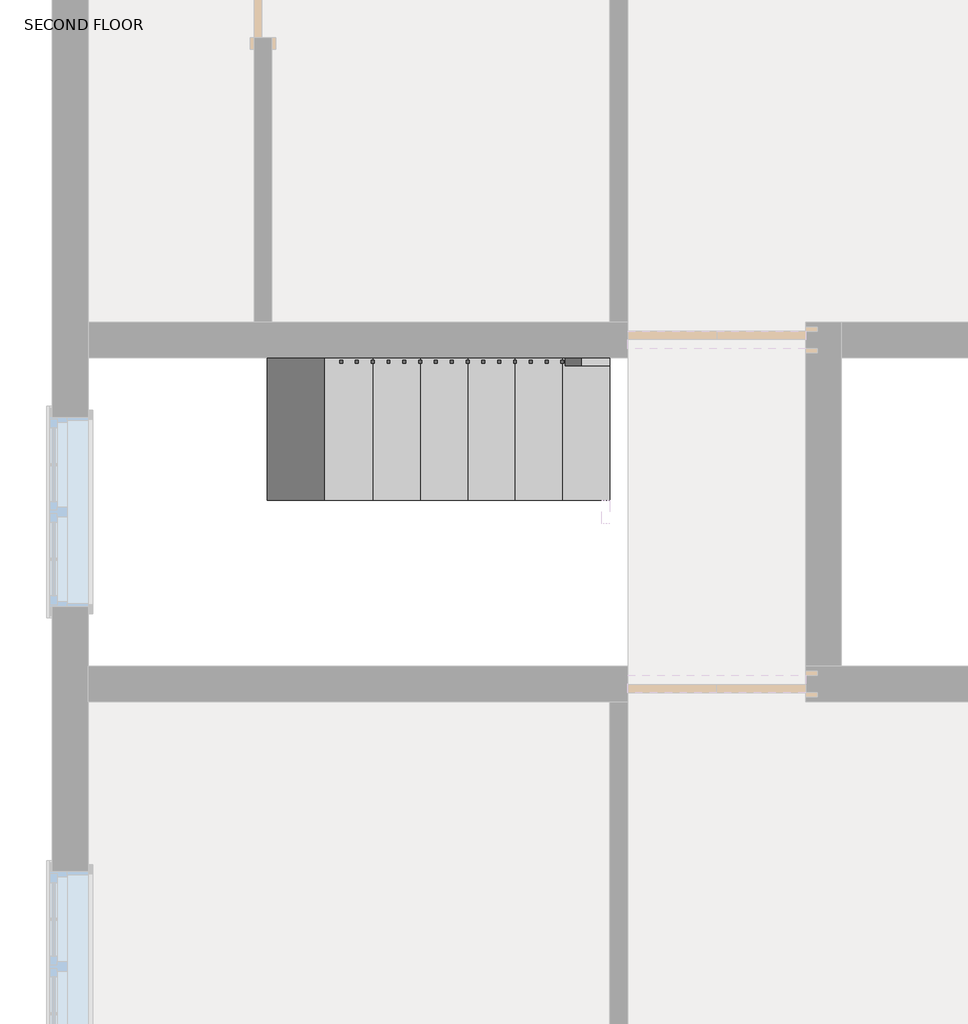
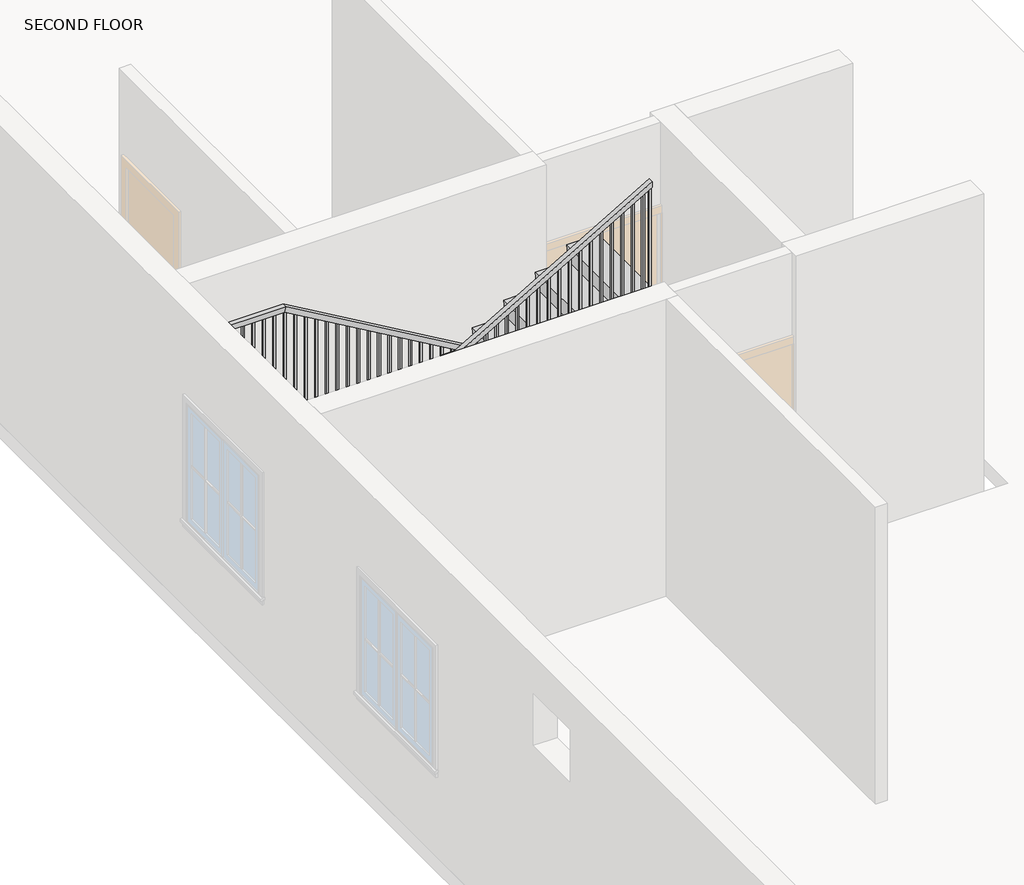
# One storey, part 3 of 4: 1 railing, 1 stair flight.
"""IFC4 building model written with IfcOpenShell, lengths in millimetres."""

from ifc_helpers import new_model, si_unit, frame, origin, place, context, project, spatial, polyline, outline, extrude, faceted_brep, element, save

model = new_model("IFC4")

# Units and contexts
model_context = context("Model", 3, world=origin())
ifc_project = project(units=[si_unit("LENGTHUNIT", "METRE", prefix="MILLI")], contexts=[model_context])

# Site, building, storey
site = spatial("IfcSite", under=ifc_project)
building = spatial("IfcBuilding", under=site)
storey = spatial("IfcBuildingStorey", under=building, Name="SECOND FLOOR", Elevation=6400.8)

# Railing
placement = place(None, origin())
element("IfcRailing", 1, ObjectType="Handrail - Rectangular", at=placement, inside=storey, context=model_context, shape_type="SolidModel", body=[
    faceted_brep([(-2776.8289041, 1499.0153263, 7493.0), (-2776.8289041, 1499.0153263, 7434.1886538), (-2776.8289041, 1549.8153263, 7434.1886538), (-2776.8289041, 1549.8153263, 7493.0), (-5215.2289041, 1499.0153263, 8915.4), (-5228.9626405, 1499.0153263, 8864.6), (-5228.9626405, 1549.8153263, 8864.6), (-5215.2289041, 1549.8153263, 8915.4), (-6078.8289041, 1499.0153263, 8915.4), (-6078.8289041, 1499.0153263, 8864.6), (-6129.6289041, 1549.8153263, 8864.6), (-6129.6289041, 1549.8153263, 8915.4), (-6078.8289041, -380.5846737, 8915.4), (-6078.8289041, -380.5846737, 8864.6), (-6129.6289041, -431.3846737, 8864.6), (-6129.6289041, -431.3846737, 8915.4), (-5520.0289041, -380.5846737, 8915.4), (-5506.2951677, -380.5846737, 8864.6), (-5506.2951677, -431.3846737, 8864.6), (-5520.0289041, -431.3846737, 8915.4), (-2776.8289041, -380.5846737, 10515.6), (-2776.8289041, -431.3846737, 10515.6), (-2776.8289041, -431.3846737, 10456.7886538), (-2776.8289041, -380.5846737, 10456.7886538)], [[[0, 1, 2, 3]], [[1, 0, 4, 5]], [[2, 1, 5, 6]], [[3, 2, 6, 7]], [[0, 3, 7, 4]], [[5, 4, 8, 9]], [[6, 5, 9, 10]], [[7, 6, 10, 11]], [[4, 7, 11, 8]], [[9, 8, 12, 13]], [[10, 9, 13, 14]], [[11, 10, 14, 15]], [[8, 11, 15, 12]], [[13, 12, 16, 17]], [[14, 13, 17, 18]], [[15, 14, 18, 19]], [[12, 15, 19, 16]], [[20, 21, 22, 23]], [[17, 16, 20, 23]], [[18, 17, 23, 22]], [[19, 18, 22, 21]], [[16, 19, 21, 20]]]),
    extrude(outline(polyline([(10417.8949038, -2843.5039041), (10406.7824038, -2862.5539041), (9423.4, -2862.5539041), (9423.4, -2843.5039041), (10417.8949038, -2843.5039041)])), frame((0.0, -415.5096737, 0.0), z_axis=(0.0, 1.0, 0.0), x_axis=(0.0, 0.0, 1.0)), (0.0, 0.0, 1.0), 19.05),
    extrude(outline(polyline([(10358.6282371, -2945.1039041), (10347.5157371, -2964.1539041), (9423.4, -2964.1539041), (9423.4, -2945.1039041), (10358.6282371, -2945.1039041)])), frame((0.0, -415.5096737, 0.0), z_axis=(0.0, 1.0, 0.0), x_axis=(0.0, 0.0, 1.0)), (0.0, 0.0, 1.0), 19.05),
    extrude(outline(polyline([(10299.3615704, -3046.7039041), (10288.2490704, -3065.7539041), (9423.4, -3065.7539041), (9423.4, -3046.7039041), (10299.3615704, -3046.7039041)])), frame((0.0, -415.5096737, 0.0), z_axis=(0.0, 1.0, 0.0), x_axis=(0.0, 0.0, 1.0)), (0.0, 0.0, 1.0), 19.05),
    extrude(outline(polyline([(10240.0949038, -3148.3039041), (10228.9824038, -3167.3539041), (9245.6, -3167.3539041), (9245.6, -3148.3039041), (10240.0949038, -3148.3039041)])), frame((0.0, -415.5096737, 0.0), z_axis=(0.0, 1.0, 0.0), x_axis=(0.0, 0.0, 1.0)), (0.0, 0.0, 1.0), 19.05),
    extrude(outline(polyline([(10180.8282371, -3249.9039041), (10169.7157371, -3268.9539041), (9245.6, -3268.9539041), (9245.6, -3249.9039041), (10180.8282371, -3249.9039041)])), frame((0.0, -415.5096737, 0.0), z_axis=(0.0, 1.0, 0.0), x_axis=(0.0, 0.0, 1.0)), (0.0, 0.0, 1.0), 19.05),
    extrude(outline(polyline([(10121.5615704, -3351.5039041), (10110.4490704, -3370.5539041), (9245.6, -3370.5539041), (9245.6, -3351.5039041), (10121.5615704, -3351.5039041)])), frame((0.0, -415.5096737, 0.0), z_axis=(0.0, 1.0, 0.0), x_axis=(0.0, 0.0, 1.0)), (0.0, 0.0, 1.0), 19.05),
    extrude(outline(polyline([(10062.2949038, -3453.1039041), (10051.1824038, -3472.1539041), (9067.8, -3472.1539041), (9067.8, -3453.1039041), (10062.2949038, -3453.1039041)])), frame((0.0, -415.5096737, 0.0), z_axis=(0.0, 1.0, 0.0), x_axis=(0.0, 0.0, 1.0)), (0.0, 0.0, 1.0), 19.05),
    extrude(outline(polyline([(10003.0282371, -3554.7039041), (9991.9157371, -3573.7539041), (9067.8, -3573.7539041), (9067.8, -3554.7039041), (10003.0282371, -3554.7039041)])), frame((0.0, -415.5096737, 0.0), z_axis=(0.0, 1.0, 0.0), x_axis=(0.0, 0.0, 1.0)), (0.0, 0.0, 1.0), 19.05),
    extrude(outline(polyline([(9943.7615704, -3656.3039041), (9932.6490704, -3675.3539041), (9067.8, -3675.3539041), (9067.8, -3656.3039041), (9943.7615704, -3656.3039041)])), frame((0.0, -415.5096737, 0.0), z_axis=(0.0, 1.0, 0.0), x_axis=(0.0, 0.0, 1.0)), (0.0, 0.0, 1.0), 19.05),
    extrude(outline(polyline([(9884.4949038, -3757.9039041), (9873.3824038, -3776.9539041), (8890.0, -3776.9539041), (8890.0, -3757.9039041), (9884.4949038, -3757.9039041)])), frame((0.0, -415.5096737, 0.0), z_axis=(0.0, 1.0, 0.0), x_axis=(0.0, 0.0, 1.0)), (0.0, 0.0, 1.0), 19.05),
    extrude(outline(polyline([(9825.2282371, -3859.5039041), (9814.1157371, -3878.5539041), (8890.0, -3878.5539041), (8890.0, -3859.5039041), (9825.2282371, -3859.5039041)])), frame((0.0, -415.5096737, 0.0), z_axis=(0.0, 1.0, 0.0), x_axis=(0.0, 0.0, 1.0)), (0.0, 0.0, 1.0), 19.05),
    extrude(outline(polyline([(9765.9615704, -3961.1039041), (9754.8490704, -3980.1539041), (8890.0, -3980.1539041), (8890.0, -3961.1039041), (9765.9615704, -3961.1039041)])), frame((0.0, -415.5096737, 0.0), z_axis=(0.0, 1.0, 0.0), x_axis=(0.0, 0.0, 1.0)), (0.0, 0.0, 1.0), 19.05),
    extrude(outline(polyline([(9706.6949038, -4062.7039041), (9695.5824038, -4081.7539041), (8712.2, -4081.7539041), (8712.2, -4062.7039041), (9706.6949038, -4062.7039041)])), frame((0.0, -415.5096737, 0.0), z_axis=(0.0, 1.0, 0.0), x_axis=(0.0, 0.0, 1.0)), (0.0, 0.0, 1.0), 19.05),
    extrude(outline(polyline([(9647.4282371, -4164.3039041), (9636.3157371, -4183.3539041), (8712.2, -4183.3539041), (8712.2, -4164.3039041), (9647.4282371, -4164.3039041)])), frame((0.0, -415.5096737, 0.0), z_axis=(0.0, 1.0, 0.0), x_axis=(0.0, 0.0, 1.0)), (0.0, 0.0, 1.0), 19.05),
    extrude(outline(polyline([(9588.1615704, -4265.9039041), (9577.0490704, -4284.9539041), (8712.2, -4284.9539041), (8712.2, -4265.9039041), (9588.1615704, -4265.9039041)])), frame((0.0, -415.5096737, 0.0), z_axis=(0.0, 1.0, 0.0), x_axis=(0.0, 0.0, 1.0)), (0.0, 0.0, 1.0), 19.05),
    extrude(outline(polyline([(9528.8949038, -4367.5039041), (9517.7824038, -4386.5539041), (8534.4, -4386.5539041), (8534.4, -4367.5039041), (9528.8949038, -4367.5039041)])), frame((0.0, -415.5096737, 0.0), z_axis=(0.0, 1.0, 0.0), x_axis=(0.0, 0.0, 1.0)), (0.0, 0.0, 1.0), 19.05),
    extrude(outline(polyline([(9469.6282371, -4469.1039041), (9458.5157371, -4488.1539041), (8534.4, -4488.1539041), (8534.4, -4469.1039041), (9469.6282371, -4469.1039041)])), frame((0.0, -415.5096737, 0.0), z_axis=(0.0, 1.0, 0.0), x_axis=(0.0, 0.0, 1.0)), (0.0, 0.0, 1.0), 19.05),
    extrude(outline(polyline([(9410.3615704, -4570.7039041), (9399.2490704, -4589.7539041), (8534.4, -4589.7539041), (8534.4, -4570.7039041), (9410.3615704, -4570.7039041)])), frame((0.0, -415.5096737, 0.0), z_axis=(0.0, 1.0, 0.0), x_axis=(0.0, 0.0, 1.0)), (0.0, 0.0, 1.0), 19.05),
    extrude(outline(polyline([(9351.0949038, -4672.3039041), (9339.9824038, -4691.3539041), (8356.6, -4691.3539041), (8356.6, -4672.3039041), (9351.0949038, -4672.3039041)])), frame((0.0, -415.5096737, 0.0), z_axis=(0.0, 1.0, 0.0), x_axis=(0.0, 0.0, 1.0)), (0.0, 0.0, 1.0), 19.05),
    extrude(outline(polyline([(9291.8282371, -4773.9039041), (9280.7157371, -4792.9539041), (8356.6, -4792.9539041), (8356.6, -4773.9039041), (9291.8282371, -4773.9039041)])), frame((0.0, -415.5096737, 0.0), z_axis=(0.0, 1.0, 0.0), x_axis=(0.0, 0.0, 1.0)), (0.0, 0.0, 1.0), 19.05),
    extrude(outline(polyline([(9232.5615704, -4875.5039041), (9221.4490704, -4894.5539041), (8356.6, -4894.5539041), (8356.6, -4875.5039041), (9232.5615704, -4875.5039041)])), frame((0.0, -415.5096737, 0.0), z_axis=(0.0, 1.0, 0.0), x_axis=(0.0, 0.0, 1.0)), (0.0, 0.0, 1.0), 19.05),
    extrude(outline(polyline([(9173.2949038, -4977.1039041), (9162.1824038, -4996.1539041), (8178.8, -4996.1539041), (8178.8, -4977.1039041), (9173.2949038, -4977.1039041)])), frame((0.0, -415.5096737, 0.0), z_axis=(0.0, 1.0, 0.0), x_axis=(0.0, 0.0, 1.0)), (0.0, 0.0, 1.0), 19.05),
    extrude(outline(polyline([(9114.0282371, -5078.7039041), (9102.9157371, -5097.7539041), (8178.8, -5097.7539041), (8178.8, -5078.7039041), (9114.0282371, -5078.7039041)])), frame((0.0, -415.5096737, 0.0), z_axis=(0.0, 1.0, 0.0), x_axis=(0.0, 0.0, 1.0)), (0.0, 0.0, 1.0), 19.05),
    extrude(outline(polyline([(9054.7615704, -5180.3039041), (9043.6490704, -5199.3539041), (8178.8, -5199.3539041), (8178.8, -5180.3039041), (9054.7615704, -5180.3039041)])), frame((0.0, -415.5096737, 0.0), z_axis=(0.0, 1.0, 0.0), x_axis=(0.0, 0.0, 1.0)), (0.0, 0.0, 1.0), 19.05),
    extrude(outline(polyline([(8995.4949038, -5281.9039041), (8984.3824038, -5300.9539041), (8001.0, -5300.9539041), (8001.0, -5281.9039041), (8995.4949038, -5281.9039041)])), frame((0.0, -415.5096737, 0.0), z_axis=(0.0, 1.0, 0.0), x_axis=(0.0, 0.0, 1.0)), (0.0, 0.0, 1.0), 19.05),
    extrude(outline(polyline([(8936.2282371, -5383.5039041), (8925.1157371, -5402.5539041), (8001.0, -5402.5539041), (8001.0, -5383.5039041), (8936.2282371, -5383.5039041)])), frame((0.0, -415.5096737, 0.0), z_axis=(0.0, 1.0, 0.0), x_axis=(0.0, 0.0, 1.0)), (0.0, 0.0, 1.0), 19.05),
    extrude(outline(polyline([(8876.9615704, -5485.1039041), (8865.8490704, -5504.1539041), (8001.0, -5504.1539041), (8001.0, -5485.1039041), (8876.9615704, -5485.1039041)])), frame((0.0, -415.5096737, 0.0), z_axis=(0.0, 1.0, 0.0), x_axis=(0.0, 0.0, 1.0)), (0.0, 0.0, 1.0), 19.05),
    extrude(outline(polyline([(-5605.7539041, -415.5096737), (-5605.7539041, -396.4596737), (-5586.7039041, -396.4596737), (-5586.7039041, -415.5096737), (-5605.7539041, -415.5096737)])), frame((0.0, 0.0, 8001.0), z_axis=(0.0, 0.0, 1.0), x_axis=(1.0, 0.0, 0.0)), (0.0, 0.0, 1.0), 863.6),
    extrude(outline(polyline([(-5707.3539041, -415.5096737), (-5707.3539041, -396.4596737), (-5688.3039041, -396.4596737), (-5688.3039041, -415.5096737), (-5707.3539041, -415.5096737)])), frame((0.0, 0.0, 8001.0), z_axis=(0.0, 0.0, 1.0), x_axis=(1.0, 0.0, 0.0)), (0.0, 0.0, 1.0), 863.6),
    extrude(outline(polyline([(-5808.9539041, -415.5096737), (-5808.9539041, -396.4596737), (-5789.9039041, -396.4596737), (-5789.9039041, -415.5096737), (-5808.9539041, -415.5096737)])), frame((0.0, 0.0, 8001.0), z_axis=(0.0, 0.0, 1.0), x_axis=(1.0, 0.0, 0.0)), (0.0, 0.0, 1.0), 863.6),
    extrude(outline(polyline([(-5910.5539041, -415.5096737), (-5910.5539041, -396.4596737), (-5891.5039041, -396.4596737), (-5891.5039041, -415.5096737), (-5910.5539041, -415.5096737)])), frame((0.0, 0.0, 8001.0), z_axis=(0.0, 0.0, 1.0), x_axis=(1.0, 0.0, 0.0)), (0.0, 0.0, 1.0), 863.6),
    extrude(outline(polyline([(-6012.1539041, -415.5096737), (-6012.1539041, -396.4596737), (-5993.1039041, -396.4596737), (-5993.1039041, -415.5096737), (-6012.1539041, -415.5096737)])), frame((0.0, 0.0, 8001.0), z_axis=(0.0, 0.0, 1.0), x_axis=(1.0, 0.0, 0.0)), (0.0, 0.0, 1.0), 863.6),
    extrude(outline(polyline([(-6113.7539041, -294.8596737), (-6094.7039041, -294.8596737), (-6094.7039041, -313.9096737), (-6113.7539041, -313.9096737), (-6113.7539041, -294.8596737)])), frame((0.0, 0.0, 8001.0), z_axis=(0.0, 0.0, 1.0), x_axis=(1.0, 0.0, 0.0)), (0.0, 0.0, 1.0), 863.6),
    extrude(outline(polyline([(-6113.7539041, -193.2596737), (-6094.7039041, -193.2596737), (-6094.7039041, -212.3096737), (-6113.7539041, -212.3096737), (-6113.7539041, -193.2596737)])), frame((0.0, 0.0, 8001.0), z_axis=(0.0, 0.0, 1.0), x_axis=(1.0, 0.0, 0.0)), (0.0, 0.0, 1.0), 863.6),
    extrude(outline(polyline([(-6113.7539041, -91.6596737), (-6094.7039041, -91.6596737), (-6094.7039041, -110.7096737), (-6113.7539041, -110.7096737), (-6113.7539041, -91.6596737)])), frame((0.0, 0.0, 8001.0), z_axis=(0.0, 0.0, 1.0), x_axis=(1.0, 0.0, 0.0)), (0.0, 0.0, 1.0), 863.6),
    extrude(outline(polyline([(-6113.7539041, 9.9403263), (-6094.7039041, 9.9403263), (-6094.7039041, -9.1096737), (-6113.7539041, -9.1096737), (-6113.7539041, 9.9403263)])), frame((0.0, 0.0, 8001.0), z_axis=(0.0, 0.0, 1.0), x_axis=(1.0, 0.0, 0.0)), (0.0, 0.0, 1.0), 863.6),
    extrude(outline(polyline([(-6113.7539041, 111.5403263), (-6094.7039041, 111.5403263), (-6094.7039041, 92.4903263), (-6113.7539041, 92.4903263), (-6113.7539041, 111.5403263)])), frame((0.0, 0.0, 8001.0), z_axis=(0.0, 0.0, 1.0), x_axis=(1.0, 0.0, 0.0)), (0.0, 0.0, 1.0), 863.6),
    extrude(outline(polyline([(-6113.7539041, 213.1403263), (-6094.7039041, 213.1403263), (-6094.7039041, 194.0903263), (-6113.7539041, 194.0903263), (-6113.7539041, 213.1403263)])), frame((0.0, 0.0, 8001.0), z_axis=(0.0, 0.0, 1.0), x_axis=(1.0, 0.0, 0.0)), (0.0, 0.0, 1.0), 863.6),
    extrude(outline(polyline([(-6113.7539041, 314.7403263), (-6094.7039041, 314.7403263), (-6094.7039041, 295.6903263), (-6113.7539041, 295.6903263), (-6113.7539041, 314.7403263)])), frame((0.0, 0.0, 8001.0), z_axis=(0.0, 0.0, 1.0), x_axis=(1.0, 0.0, 0.0)), (0.0, 0.0, 1.0), 863.6),
    extrude(outline(polyline([(-6113.7539041, 416.3403263), (-6094.7039041, 416.3403263), (-6094.7039041, 397.2903263), (-6113.7539041, 397.2903263), (-6113.7539041, 416.3403263)])), frame((0.0, 0.0, 8001.0), z_axis=(0.0, 0.0, 1.0), x_axis=(1.0, 0.0, 0.0)), (0.0, 0.0, 1.0), 863.6),
    extrude(outline(polyline([(-6113.7539041, 517.9403263), (-6094.7039041, 517.9403263), (-6094.7039041, 498.8903263), (-6113.7539041, 498.8903263), (-6113.7539041, 517.9403263)])), frame((0.0, 0.0, 8001.0), z_axis=(0.0, 0.0, 1.0), x_axis=(1.0, 0.0, 0.0)), (0.0, 0.0, 1.0), 863.6),
    extrude(outline(polyline([(-6113.7539041, 619.5403263), (-6094.7039041, 619.5403263), (-6094.7039041, 600.4903263), (-6113.7539041, 600.4903263), (-6113.7539041, 619.5403263)])), frame((0.0, 0.0, 8001.0), z_axis=(0.0, 0.0, 1.0), x_axis=(1.0, 0.0, 0.0)), (0.0, 0.0, 1.0), 863.6),
    extrude(outline(polyline([(-6113.7539041, 721.1403263), (-6094.7039041, 721.1403263), (-6094.7039041, 702.0903263), (-6113.7539041, 702.0903263), (-6113.7539041, 721.1403263)])), frame((0.0, 0.0, 8001.0), z_axis=(0.0, 0.0, 1.0), x_axis=(1.0, 0.0, 0.0)), (0.0, 0.0, 1.0), 863.6),
    extrude(outline(polyline([(-6113.7539041, 822.7403263), (-6094.7039041, 822.7403263), (-6094.7039041, 803.6903263), (-6113.7539041, 803.6903263), (-6113.7539041, 822.7403263)])), frame((0.0, 0.0, 8001.0), z_axis=(0.0, 0.0, 1.0), x_axis=(1.0, 0.0, 0.0)), (0.0, 0.0, 1.0), 863.6),
    extrude(outline(polyline([(-6113.7539041, 924.3403263), (-6094.7039041, 924.3403263), (-6094.7039041, 905.2903263), (-6113.7539041, 905.2903263), (-6113.7539041, 924.3403263)])), frame((0.0, 0.0, 8001.0), z_axis=(0.0, 0.0, 1.0), x_axis=(1.0, 0.0, 0.0)), (0.0, 0.0, 1.0), 863.6),
    extrude(outline(polyline([(-6113.7539041, 1025.9403263), (-6094.7039041, 1025.9403263), (-6094.7039041, 1006.8903263), (-6113.7539041, 1006.8903263), (-6113.7539041, 1025.9403263)])), frame((0.0, 0.0, 8001.0), z_axis=(0.0, 0.0, 1.0), x_axis=(1.0, 0.0, 0.0)), (0.0, 0.0, 1.0), 863.6),
    extrude(outline(polyline([(-6113.7539041, 1127.5403263), (-6094.7039041, 1127.5403263), (-6094.7039041, 1108.4903263), (-6113.7539041, 1108.4903263), (-6113.7539041, 1127.5403263)])), frame((0.0, 0.0, 8001.0), z_axis=(0.0, 0.0, 1.0), x_axis=(1.0, 0.0, 0.0)), (0.0, 0.0, 1.0), 863.6),
    extrude(outline(polyline([(-6113.7539041, 1229.1403263), (-6094.7039041, 1229.1403263), (-6094.7039041, 1210.0903263), (-6113.7539041, 1210.0903263), (-6113.7539041, 1229.1403263)])), frame((0.0, 0.0, 8001.0), z_axis=(0.0, 0.0, 1.0), x_axis=(1.0, 0.0, 0.0)), (0.0, 0.0, 1.0), 863.6),
    extrude(outline(polyline([(-6113.7539041, 1330.7403263), (-6094.7039041, 1330.7403263), (-6094.7039041, 1311.6903263), (-6113.7539041, 1311.6903263), (-6113.7539041, 1330.7403263)])), frame((0.0, 0.0, 8001.0), z_axis=(0.0, 0.0, 1.0), x_axis=(1.0, 0.0, 0.0)), (0.0, 0.0, 1.0), 863.6),
    extrude(outline(polyline([(-6113.7539041, 1432.3403263), (-6094.7039041, 1432.3403263), (-6094.7039041, 1413.2903263), (-6113.7539041, 1413.2903263), (-6113.7539041, 1432.3403263)])), frame((0.0, 0.0, 8001.0), z_axis=(0.0, 0.0, 1.0), x_axis=(1.0, 0.0, 0.0)), (0.0, 0.0, 1.0), 863.6),
    extrude(outline(polyline([(-6018.5039041, 1533.9403263), (-6018.5039041, 1514.8903263), (-6037.5539041, 1514.8903263), (-6037.5539041, 1533.9403263), (-6018.5039041, 1533.9403263)])), frame((0.0, 0.0, 8001.0), z_axis=(0.0, 0.0, 1.0), x_axis=(1.0, 0.0, 0.0)), (0.0, 0.0, 1.0), 863.6),
    extrude(outline(polyline([(-5916.9039041, 1533.9403263), (-5916.9039041, 1514.8903263), (-5935.9539041, 1514.8903263), (-5935.9539041, 1533.9403263), (-5916.9039041, 1533.9403263)])), frame((0.0, 0.0, 8001.0), z_axis=(0.0, 0.0, 1.0), x_axis=(1.0, 0.0, 0.0)), (0.0, 0.0, 1.0), 863.6),
    extrude(outline(polyline([(-5815.3039041, 1533.9403263), (-5815.3039041, 1514.8903263), (-5834.3539041, 1514.8903263), (-5834.3539041, 1533.9403263), (-5815.3039041, 1533.9403263)])), frame((0.0, 0.0, 8001.0), z_axis=(0.0, 0.0, 1.0), x_axis=(1.0, 0.0, 0.0)), (0.0, 0.0, 1.0), 863.6),
    extrude(outline(polyline([(-5713.7039041, 1533.9403263), (-5713.7039041, 1514.8903263), (-5732.7539041, 1514.8903263), (-5732.7539041, 1533.9403263), (-5713.7039041, 1533.9403263)])), frame((0.0, 0.0, 8001.0), z_axis=(0.0, 0.0, 1.0), x_axis=(1.0, 0.0, 0.0)), (0.0, 0.0, 1.0), 863.6),
    extrude(outline(polyline([(-5612.1039041, 1533.9403263), (-5612.1039041, 1514.8903263), (-5631.1539041, 1514.8903263), (-5631.1539041, 1533.9403263), (-5612.1039041, 1533.9403263)])), frame((0.0, 0.0, 8001.0), z_axis=(0.0, 0.0, 1.0), x_axis=(1.0, 0.0, 0.0)), (0.0, 0.0, 1.0), 863.6),
    extrude(outline(polyline([(-5510.5039041, 1533.9403263), (-5510.5039041, 1514.8903263), (-5529.5539041, 1514.8903263), (-5529.5539041, 1533.9403263), (-5510.5039041, 1533.9403263)])), frame((0.0, 0.0, 8001.0), z_axis=(0.0, 0.0, 1.0), x_axis=(1.0, 0.0, 0.0)), (0.0, 0.0, 1.0), 863.6),
    extrude(outline(polyline([(-5408.9039041, 1533.9403263), (-5408.9039041, 1514.8903263), (-5427.9539041, 1514.8903263), (-5427.9539041, 1533.9403263), (-5408.9039041, 1533.9403263)])), frame((0.0, 0.0, 8001.0), z_axis=(0.0, 0.0, 1.0), x_axis=(1.0, 0.0, 0.0)), (0.0, 0.0, 1.0), 863.6),
    extrude(outline(polyline([(-5307.3039041, 1533.9403263), (-5307.3039041, 1514.8903263), (-5326.3539041, 1514.8903263), (-5326.3539041, 1533.9403263), (-5307.3039041, 1533.9403263)])), frame((0.0, 0.0, 8001.0), z_axis=(0.0, 0.0, 1.0), x_axis=(1.0, 0.0, 0.0)), (0.0, 0.0, 1.0), 863.6),
    extrude(outline(polyline([(8851.0324038, -5205.7039041), (8862.1449038, -5224.7539041), (8001.0, -5224.7539041), (8001.0, -5205.7039041), (8851.0324038, -5205.7039041)])), frame((0.0, 1514.8903263, 0.0), z_axis=(0.0, 1.0, 0.0), x_axis=(0.0, 0.0, 1.0)), (0.0, 0.0, 1.0), 19.05),
    extrude(outline(polyline([(8791.7657371, -5104.1039041), (8802.8782371, -5123.1539041), (7823.2, -5123.1539041), (7823.2, -5104.1039041), (8791.7657371, -5104.1039041)])), frame((0.0, 1514.8903263, 0.0), z_axis=(0.0, 1.0, 0.0), x_axis=(0.0, 0.0, 1.0)), (0.0, 0.0, 1.0), 19.05),
    extrude(outline(polyline([(8732.4990704, -5002.5039041), (8743.6115704, -5021.5539041), (7823.2, -5021.5539041), (7823.2, -5002.5039041), (8732.4990704, -5002.5039041)])), frame((0.0, 1514.8903263, 0.0), z_axis=(0.0, 1.0, 0.0), x_axis=(0.0, 0.0, 1.0)), (0.0, 0.0, 1.0), 19.05),
    extrude(outline(polyline([(8673.2324038, -4900.9039041), (8684.3449038, -4919.9539041), (7823.2, -4919.9539041), (7823.2, -4900.9039041), (8673.2324038, -4900.9039041)])), frame((0.0, 1514.8903263, 0.0), z_axis=(0.0, 1.0, 0.0), x_axis=(0.0, 0.0, 1.0)), (0.0, 0.0, 1.0), 19.05),
    extrude(outline(polyline([(8613.9657371, -4799.3039041), (8625.0782371, -4818.3539041), (7645.4, -4818.3539041), (7645.4, -4799.3039041), (8613.9657371, -4799.3039041)])), frame((0.0, 1514.8903263, 0.0), z_axis=(0.0, 1.0, 0.0), x_axis=(0.0, 0.0, 1.0)), (0.0, 0.0, 1.0), 19.05),
    extrude(outline(polyline([(8554.6990704, -4697.7039041), (8565.8115704, -4716.7539041), (7645.4, -4716.7539041), (7645.4, -4697.7039041), (8554.6990704, -4697.7039041)])), frame((0.0, 1514.8903263, 0.0), z_axis=(0.0, 1.0, 0.0), x_axis=(0.0, 0.0, 1.0)), (0.0, 0.0, 1.0), 19.05),
    extrude(outline(polyline([(8495.4324038, -4596.1039041), (8506.5449038, -4615.1539041), (7645.4, -4615.1539041), (7645.4, -4596.1039041), (8495.4324038, -4596.1039041)])), frame((0.0, 1514.8903263, 0.0), z_axis=(0.0, 1.0, 0.0), x_axis=(0.0, 0.0, 1.0)), (0.0, 0.0, 1.0), 19.05),
    extrude(outline(polyline([(8436.1657371, -4494.5039041), (8447.2782371, -4513.5539041), (7467.6, -4513.5539041), (7467.6, -4494.5039041), (8436.1657371, -4494.5039041)])), frame((0.0, 1514.8903263, 0.0), z_axis=(0.0, 1.0, 0.0), x_axis=(0.0, 0.0, 1.0)), (0.0, 0.0, 1.0), 19.05),
    extrude(outline(polyline([(8376.8990704, -4392.9039041), (8388.0115704, -4411.9539041), (7467.6, -4411.9539041), (7467.6, -4392.9039041), (8376.8990704, -4392.9039041)])), frame((0.0, 1514.8903263, 0.0), z_axis=(0.0, 1.0, 0.0), x_axis=(0.0, 0.0, 1.0)), (0.0, 0.0, 1.0), 19.05),
    extrude(outline(polyline([(8317.6324038, -4291.3039041), (8328.7449038, -4310.3539041), (7467.6, -4310.3539041), (7467.6, -4291.3039041), (8317.6324038, -4291.3039041)])), frame((0.0, 1514.8903263, 0.0), z_axis=(0.0, 1.0, 0.0), x_axis=(0.0, 0.0, 1.0)), (0.0, 0.0, 1.0), 19.05),
    extrude(outline(polyline([(8258.3657371, -4189.7039041), (8269.4782371, -4208.7539041), (7289.8, -4208.7539041), (7289.8, -4189.7039041), (8258.3657371, -4189.7039041)])), frame((0.0, 1514.8903263, 0.0), z_axis=(0.0, 1.0, 0.0), x_axis=(0.0, 0.0, 1.0)), (0.0, 0.0, 1.0), 19.05),
    extrude(outline(polyline([(8199.0990704, -4088.1039041), (8210.2115704, -4107.1539041), (7289.8, -4107.1539041), (7289.8, -4088.1039041), (8199.0990704, -4088.1039041)])), frame((0.0, 1514.8903263, 0.0), z_axis=(0.0, 1.0, 0.0), x_axis=(0.0, 0.0, 1.0)), (0.0, 0.0, 1.0), 19.05),
    extrude(outline(polyline([(8139.8324038, -3986.5039041), (8150.9449038, -4005.5539041), (7289.8, -4005.5539041), (7289.8, -3986.5039041), (8139.8324038, -3986.5039041)])), frame((0.0, 1514.8903263, 0.0), z_axis=(0.0, 1.0, 0.0), x_axis=(0.0, 0.0, 1.0)), (0.0, 0.0, 1.0), 19.05),
    extrude(outline(polyline([(8080.5657371, -3884.9039041), (8091.6782371, -3903.9539041), (7112.0, -3903.9539041), (7112.0, -3884.9039041), (8080.5657371, -3884.9039041)])), frame((0.0, 1514.8903263, 0.0), z_axis=(0.0, 1.0, 0.0), x_axis=(0.0, 0.0, 1.0)), (0.0, 0.0, 1.0), 19.05),
    extrude(outline(polyline([(8021.2990704, -3783.3039041), (8032.4115704, -3802.3539041), (7112.0, -3802.3539041), (7112.0, -3783.3039041), (8021.2990704, -3783.3039041)])), frame((0.0, 1514.8903263, 0.0), z_axis=(0.0, 1.0, 0.0), x_axis=(0.0, 0.0, 1.0)), (0.0, 0.0, 1.0), 19.05),
    extrude(outline(polyline([(7962.0324038, -3681.7039041), (7973.1449038, -3700.7539041), (7112.0, -3700.7539041), (7112.0, -3681.7039041), (7962.0324038, -3681.7039041)])), frame((0.0, 1514.8903263, 0.0), z_axis=(0.0, 1.0, 0.0), x_axis=(0.0, 0.0, 1.0)), (0.0, 0.0, 1.0), 19.05),
    extrude(outline(polyline([(7902.7657371, -3580.1039041), (7913.8782371, -3599.1539041), (6934.2, -3599.1539041), (6934.2, -3580.1039041), (7902.7657371, -3580.1039041)])), frame((0.0, 1514.8903263, 0.0), z_axis=(0.0, 1.0, 0.0), x_axis=(0.0, 0.0, 1.0)), (0.0, 0.0, 1.0), 19.05),
    extrude(outline(polyline([(7843.4990704, -3478.5039041), (7854.6115704, -3497.5539041), (6934.2, -3497.5539041), (6934.2, -3478.5039041), (7843.4990704, -3478.5039041)])), frame((0.0, 1514.8903263, 0.0), z_axis=(0.0, 1.0, 0.0), x_axis=(0.0, 0.0, 1.0)), (0.0, 0.0, 1.0), 19.05),
    extrude(outline(polyline([(7784.2324038, -3376.9039041), (7795.3449038, -3395.9539041), (6934.2, -3395.9539041), (6934.2, -3376.9039041), (7784.2324038, -3376.9039041)])), frame((0.0, 1514.8903263, 0.0), z_axis=(0.0, 1.0, 0.0), x_axis=(0.0, 0.0, 1.0)), (0.0, 0.0, 1.0), 19.05),
    extrude(outline(polyline([(7724.9657371, -3275.3039041), (7736.0782371, -3294.3539041), (6756.4, -3294.3539041), (6756.4, -3275.3039041), (7724.9657371, -3275.3039041)])), frame((0.0, 1514.8903263, 0.0), z_axis=(0.0, 1.0, 0.0), x_axis=(0.0, 0.0, 1.0)), (0.0, 0.0, 1.0), 19.05),
    extrude(outline(polyline([(7665.6990704, -3173.7039041), (7676.8115704, -3192.7539041), (6756.4, -3192.7539041), (6756.4, -3173.7039041), (7665.6990704, -3173.7039041)])), frame((0.0, 1514.8903263, 0.0), z_axis=(0.0, 1.0, 0.0), x_axis=(0.0, 0.0, 1.0)), (0.0, 0.0, 1.0), 19.05),
    extrude(outline(polyline([(7606.4324038, -3072.1039041), (7617.5449038, -3091.1539041), (6756.4, -3091.1539041), (6756.4, -3072.1039041), (7606.4324038, -3072.1039041)])), frame((0.0, 1514.8903263, 0.0), z_axis=(0.0, 1.0, 0.0), x_axis=(0.0, 0.0, 1.0)), (0.0, 0.0, 1.0), 19.05),
    extrude(outline(polyline([(7547.1657371, -2970.5039041), (7558.2782371, -2989.5539041), (6578.6, -2989.5539041), (6578.6, -2970.5039041), (7547.1657371, -2970.5039041)])), frame((0.0, 1514.8903263, 0.0), z_axis=(0.0, 1.0, 0.0), x_axis=(0.0, 0.0, 1.0)), (0.0, 0.0, 1.0), 19.05),
    extrude(outline(polyline([(7487.8990704, -2868.9039041), (7499.0115704, -2887.9539041), (6578.6, -2887.9539041), (6578.6, -2868.9039041), (7487.8990704, -2868.9039041)])), frame((0.0, 1514.8903263, 0.0), z_axis=(0.0, 1.0, 0.0), x_axis=(0.0, 0.0, 1.0)), (0.0, 0.0, 1.0), 19.05),
    extrude(outline(polyline([(-6113.7539041, -396.4596737), (-6094.7039041, -396.4596737), (-6094.7039041, -415.5096737), (-6113.7539041, -415.5096737), (-6113.7539041, -396.4596737)])), frame((0.0, 0.0, 8001.0), z_axis=(0.0, 0.0, 1.0), x_axis=(1.0, 0.0, 0.0)), (0.0, 0.0, 1.0), 863.6),
    extrude(outline(polyline([(-6094.7039041, 1533.9403263), (-6094.7039041, 1514.8903263), (-6113.7539041, 1514.8903263), (-6113.7539041, 1533.9403263), (-6094.7039041, 1533.9403263)])), frame((0.0, 0.0, 8001.0), z_axis=(0.0, 0.0, 1.0), x_axis=(1.0, 0.0, 0.0)), (0.0, 0.0, 1.0), 863.6),
    extrude(outline(polyline([(10456.7886538, -2776.8289041), (10445.6761538, -2795.8789041), (9423.4, -2795.8789041), (9423.4, -2776.8289041), (10456.7886538, -2776.8289041)])), frame((0.0, -415.5096737, 0.0), z_axis=(0.0, 1.0, 0.0), x_axis=(0.0, 0.0, 1.0)), (0.0, 0.0, 1.0), 19.05),
    extrude(outline(polyline([(7434.1886538, -2776.8289041), (7445.3011538, -2795.8789041), (6578.6, -2795.8789041), (6578.6, -2776.8289041), (7434.1886538, -2776.8289041)])), frame((0.0, 1514.8903263, 0.0), z_axis=(0.0, 1.0, 0.0), x_axis=(0.0, 0.0, 1.0)), (0.0, 0.0, 1.0), 19.05),
])

# Stair flight
element("IfcStairFlight", 2, ObjectType="3/4\" Nosing", at=placement, inside=storey, context=model_context, shape_type="Brep", body=[
    faceted_brep([(-2776.8289041, 635.4153263, 6578.6), (-2776.8289041, 1549.8153263, 6578.6), (-3100.6789041, 1549.8153263, 6578.6), (-3100.6789041, 635.4153263, 6578.6), (-3100.6789041, 635.4153263, 6505.0858172), (-2921.9032174, 635.4153263, 6400.8), (-2795.8789041, 635.4153263, 6400.8), (-2795.8789041, 1549.8153263, 6400.8), (-2921.9032174, 1549.8153263, 6400.8), (-3100.6789041, 1549.8153263, 6505.0858172), (-3081.6289041, 635.4153263, 6756.4), (-3081.6289041, 1549.8153263, 6756.4), (-3405.4789041, 1549.8153263, 6756.4), (-3405.4789041, 635.4153263, 6756.4), (-3405.4789041, 635.4153263, 6682.8858172), (-3405.4789041, 1549.8153263, 6682.8858172), (-3386.4289041, 635.4153263, 6934.2), (-3386.4289041, 1549.8153263, 6934.2), (-3710.2789041, 1549.8153263, 6934.2), (-3710.2789041, 635.4153263, 6934.2), (-3710.2789041, 635.4153263, 6860.6858172), (-3710.2789041, 1549.8153263, 6860.6858172), (-3691.2289041, 635.4153263, 7112.0), (-3691.2289041, 1549.8153263, 7112.0), (-4015.0789041, 1549.8153263, 7112.0), (-4015.0789041, 635.4153263, 7112.0), (-4015.0789041, 635.4153263, 7038.4858172), (-4015.0789041, 1549.8153263, 7038.4858172), (-3996.0289041, 635.4153263, 7289.8), (-3996.0289041, 1549.8153263, 7289.8), (-4319.8789041, 1549.8153263, 7289.8), (-4319.8789041, 635.4153263, 7289.8), (-4300.8289041, 635.4153263, 7467.6), (-4624.6789041, 635.4153263, 7467.6), (-4605.6289041, 635.4153263, 7645.4), (-4929.4789041, 635.4153263, 7645.4), (-4910.4289041, 635.4153263, 7823.2), (-5234.2789041, 635.4153263, 7823.2), (-5222.0324755, 635.4153263, 7937.5), (-5556.2460745, 635.4153263, 7937.5), (-4319.8789041, 1549.8153263, 7216.2858172), (-4300.8289041, 1549.8153263, 7467.6), (-4624.6789041, 1549.8153263, 7467.6), (-4624.6789041, 1549.8153263, 7394.0858172), (-4605.6289041, 1549.8153263, 7645.4), (-4929.4789041, 1549.8153263, 7645.4), (-4929.4789041, 1549.8153263, 7571.8858172), (-4910.4289041, 1549.8153263, 7823.2), (-5234.2789041, 1549.8153263, 7823.2), (-5234.2789041, 1549.8153263, 7749.6858172), (-5070.1545907, 483.0153263, 8001.0), (-2776.8289041, 483.0153263, 8001.0), (-2776.8289041, 635.4153263, 8001.0), (-3836.3032174, 635.4153263, 8001.0), (-5215.2289041, 635.4153263, 8001.0), (-5215.2289041, 1549.8153263, 8001.0), (-5556.2460745, 1549.8153263, 8001.0), (-6129.6289041, 1549.8153263, 8001.0), (-6129.6289041, -431.3846737, 8001.0), (-5196.1789041, -431.3846737, 8001.0), (-5196.1789041, 483.0153263, 8001.0), (-5179.0117336, 483.0153263, 7937.5), (-2776.8289041, 483.0153263, 7937.5), (-2776.8289041, 635.4153263, 7937.5), (-3727.4460745, 635.4153263, 7937.5), (-5556.2460745, 1549.8153263, 7937.5), (-6129.6289041, 1549.8153263, 7937.5), (-6129.6289041, -431.3846737, 7937.5), (-5196.1789041, -431.3846737, 7937.5), (-5215.2289041, 483.0153263, 8178.8), (-5215.2289041, -431.3846737, 8178.8), (-5179.0117336, -431.3846737, 8178.8), (-4891.3789041, -431.3846737, 8178.8), (-4891.3789041, 483.0153263, 8178.8), (-4891.3789041, 483.0153263, 8105.2858172), (-5179.0117336, -431.3846737, 7937.5), (-4891.3789041, -431.3846737, 8105.2858172), (-4910.4289041, 483.0153263, 8356.6), (-4910.4289041, -431.3846737, 8356.6), (-4586.5789041, -431.3846737, 8356.6), (-4586.5789041, 483.0153263, 8356.6), (-4586.5789041, 483.0153263, 8283.0858172), (-4586.5789041, -431.3846737, 8283.0858172), (-4605.6289041, 483.0153263, 8534.4), (-4605.6289041, -431.3846737, 8534.4), (-4281.7789041, -431.3846737, 8534.4), (-4281.7789041, 483.0153263, 8534.4), (-4281.7789041, 483.0153263, 8470.9), (-4281.7789041, 483.0153263, 8460.8858172), (-4598.8253326, 483.0153263, 8470.9), (-4281.7789041, -431.3846737, 8460.8858172), (-4300.8289041, 483.0153263, 8712.2), (-4300.8289041, -431.3846737, 8712.2), (-3976.9789041, -431.3846737, 8712.2), (-3976.9789041, 483.0153263, 8712.2), (-3976.9789041, 483.0153263, 8638.6858172), (-4264.6117336, 483.0153263, 8470.9), (-3976.9789041, -431.3846737, 8638.6858172), (-3996.0289041, 483.0153263, 8890.0), (-3996.0289041, -431.3846737, 8890.0), (-3672.1789041, -431.3846737, 8890.0), (-3672.1789041, 483.0153263, 8890.0), (-3672.1789041, 483.0153263, 8816.4858172), (-3672.1789041, -431.3846737, 8816.4858172), (-3691.2289041, 483.0153263, 9067.8), (-3691.2289041, -431.3846737, 9067.8), (-3367.3789041, -431.3846737, 9067.8), (-3367.3789041, 483.0153263, 9067.8), (-3367.3789041, 483.0153263, 8994.2858172), (-3367.3789041, -431.3846737, 8994.2858172), (-3386.4289041, 483.0153263, 9245.6), (-3386.4289041, -431.3846737, 9245.6), (-3062.5789041, -431.3846737, 9245.6), (-3062.5789041, 483.0153263, 9245.6), (-3062.5789041, 483.0153263, 9172.0858172), (-3062.5789041, -431.3846737, 9172.0858172), (-3081.6289041, 483.0153263, 9423.4), (-3081.6289041, -431.3846737, 9423.4), (-2776.8289041, -431.3846737, 9423.4), (-2776.8289041, 483.0153263, 9423.4), (-2776.8289041, 483.0153263, 9338.7733172), (-2776.8289041, -431.3846737, 9338.7733172)], [[[0, 1, 2, 3]], [[0, 3, 4, 5, 6]], [[2, 1, 7, 8, 9]], [[10, 11, 12, 13]], [[10, 13, 14, 4, 3]], [[12, 11, 2, 9, 15]], [[16, 17, 18, 19]], [[16, 19, 20, 14, 13]], [[18, 17, 12, 15, 21]], [[22, 23, 24, 25]], [[22, 25, 26, 20, 19]], [[24, 23, 18, 21, 27]], [[28, 29, 30, 31]], [[26, 25, 28, 31, 32, 33, 34, 35, 36, 37, 38, 39]], [[30, 29, 24, 27, 40]], [[32, 41, 42, 33]], [[42, 41, 30, 40, 43]], [[34, 44, 45, 35]], [[45, 44, 42, 43, 46]], [[36, 47, 48, 37]], [[48, 47, 45, 46, 49]], [[50, 51, 52, 53, 54, 55, 56, 57, 58, 59, 60]], [[50, 61, 62, 51]], [[52, 51, 62, 63]], [[52, 63, 64, 38, 54, 53]], [[55, 48, 49, 65, 66, 57, 56]], [[58, 57, 66, 67]], [[59, 58, 67, 68]], [[69, 70, 71, 72, 73]], [[69, 73, 74, 50, 60]], [[70, 59, 68, 75, 76, 72, 71]], [[77, 78, 79, 80]], [[77, 80, 81, 74, 73]], [[79, 78, 72, 76, 82]], [[83, 84, 85, 86]], [[83, 86, 87, 88, 81, 80, 89]], [[85, 84, 79, 82, 90]], [[91, 92, 93, 94]], [[91, 94, 95, 96, 88, 87, 86]], [[93, 92, 85, 90, 97]], [[98, 99, 100, 101]], [[98, 101, 102, 95, 94]], [[100, 99, 93, 97, 103]], [[104, 105, 106, 107]], [[104, 107, 108, 102, 101]], [[106, 105, 100, 103, 109]], [[110, 111, 112, 113]], [[110, 113, 114, 108, 107]], [[112, 111, 106, 109, 115]], [[1, 0, 6, 7]], [[3, 2, 11, 10]], [[13, 12, 17, 16]], [[19, 18, 23, 22]], [[25, 24, 29, 28]], [[31, 30, 41, 32]], [[33, 42, 44, 34]], [[35, 45, 47, 36]], [[37, 48, 55, 54, 38]], [[60, 59, 70, 69]], [[73, 72, 78, 77]], [[80, 79, 84, 83, 89]], [[86, 85, 92, 91]], [[94, 93, 99, 98]], [[101, 100, 105, 104]], [[107, 106, 111, 110]], [[116, 117, 118, 119]], [[116, 119, 120, 114, 113]], [[118, 117, 112, 115, 121]], [[119, 118, 121, 120]], [[113, 112, 117, 116]], [[7, 6, 5, 8]], [[26, 39, 65, 49, 46, 43, 40, 27, 21, 15, 9, 8, 5, 4, 14, 20]], [[65, 39, 38, 64, 63, 62, 61, 75, 68, 67, 66]], [[75, 61, 50, 74, 81, 88, 96, 95, 102, 108, 114, 120, 121, 115, 109, 103, 97, 90, 82, 76]]]),
])

save(model, "model.ifc")

# Revit data of these elements
# Type "Handrail - Rectangular"
#   Assembly Code = "C2010400"
#   built-in parameter 1008612 = 0.0416667 (stored number, unit not read)
#   built-in parameter 1008611 = 0.0416667 (stored number, unit not read)
#   built-in parameter 1008609 = 0.333333 (stored number, unit not read)
#   built-in parameter 1008604 = 0.166667 (stored number, unit not read)
#   built-in parameter 1008603 = 0.166667 (stored number, unit not read)
#   Railing Height = 3' - 0"
#   built-in parameter 1008630 = 2
#   built-in parameter 1008610 = 2
#   built-in parameter 1008618 = Baluster - Square : 3/4"
# Element 1 (IfcRailing, "Handrail - Rectangular")
#   Phase Created = New Construction
# Element 2 (IfcStairFlight, "3/4\" Nosing")
#   Phase Created = New Construction
#   Materials on its faces: "Concrete, Cast-in-Place gray"
# Materials
#   "Concrete, Cast-in-Place gray": class "Concrete", colour RGB 192 192 192, transparency 0, Description = "Cast-in-place concrete", Cost = 0
